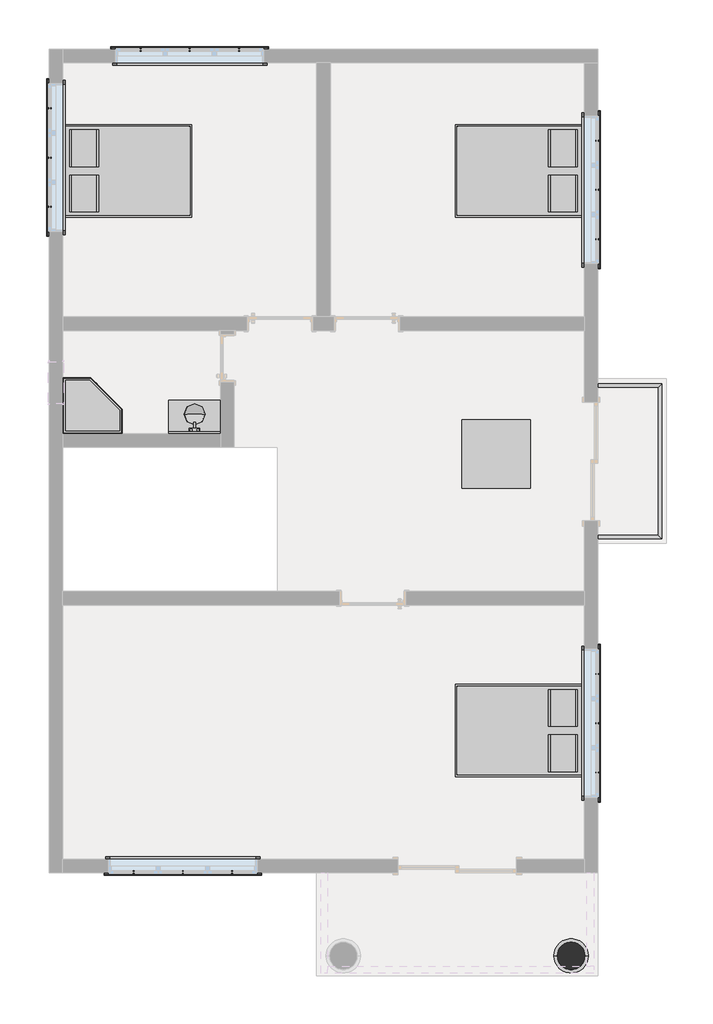
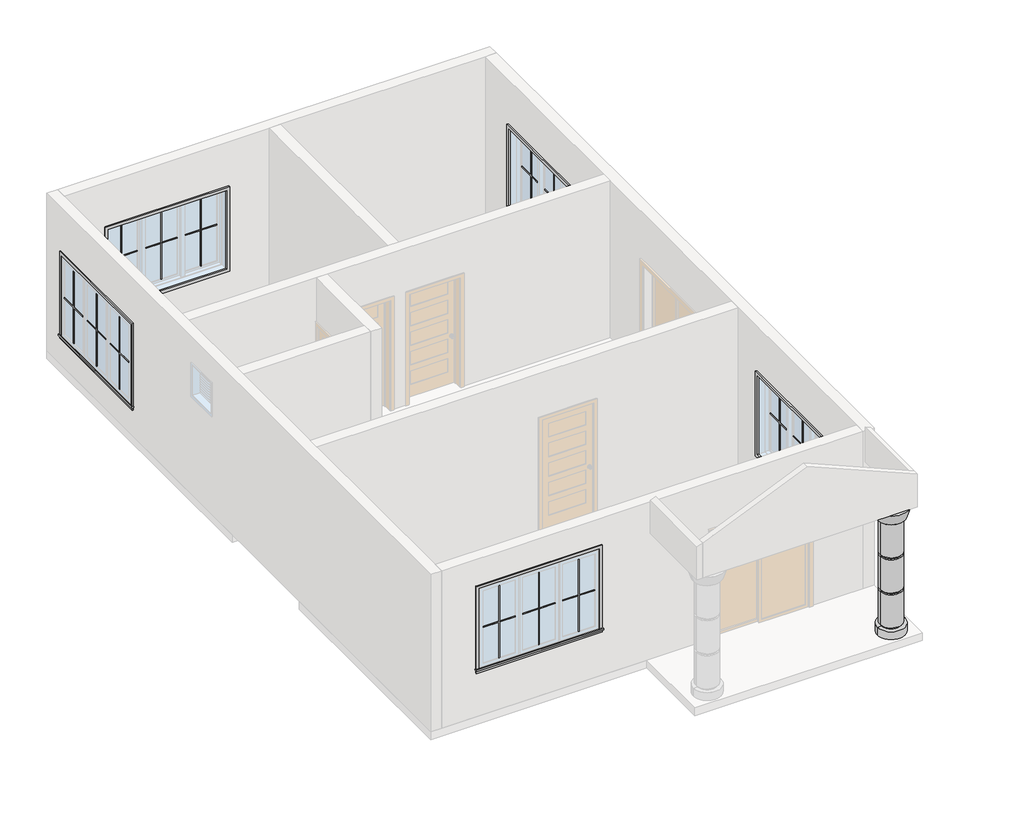
# One storey, part 2 of 2: 25 proxies, 4 furniture elements, 2 flow terminals, 1 column, 1 railing.
"""IFC4 building model written with IfcOpenShell, lengths in millimetres."""

from ifc_helpers import new_model, si_unit, frame, origin, place, context, project, spatial, polyline, circle_curve, outline, extrude, faceted_brep, transform, mapped, element, save
from ifc_brep_helpers import plane_surface, cylinder_surface, revolved_surface, advanced_brep
from components import muntin_pattern_2x2_muntin_pattern_2x2_6849e3ed, muntin_pattern_2x2_muntin_pattern_2x2_a6c43cb1, trim_window_exterior_flat_with_sill_088bf4ff, trim_window_interior_flat_picture_frame_12843d3c, flow_terminal_15267b2a, flow_terminal_2596653b, furniture_1000_x_1000mm_85c88e14, furniture_b58f7881

model = new_model("IFC4")

# Units and contexts
model_context = context("Model", 3, world=origin())
ifc_project = project(units=[si_unit("LENGTHUNIT", "METRE", prefix="MILLI")], contexts=[model_context])

# Site, building, storey
site = spatial("IfcSite", under=ifc_project)
building = spatial("IfcBuilding", under=site)
storey = spatial("IfcBuildingStorey", under=building, Elevation=3400.0)

# Proxies
placement = place(None, origin())
muntin_pattern_2x2_muntin_pattern_2x2_shape = muntin_pattern_2x2_muntin_pattern_2x2_6849e3ed(model_context)
element("IfcBuildingElementProxy", 1, Name="Muntin Pattern_2x2 : Muntin Pattern_2x2", ObjectType="Muntin Pattern_2x2 : Muntin Pattern_2x2", at=placement, inside=storey, context=model_context, shape_type="MappedRepresentation", body=[
    mapped(muntin_pattern_2x2_muntin_pattern_2x2_shape, transform((2649.7091997, -1368.0932863, 4058.55), x_axis=(0.0, -1.0, 0.0), y_axis=(1.0, 0.0, 0.0), z_axis=(0.0, 0.0, 1.0))),
])
element("IfcBuildingElementProxy", 2, Name="Muntin Pattern_2x2 : Muntin Pattern_2x2", ObjectType="Muntin Pattern_2x2 : Muntin Pattern_2x2", at=placement, inside=storey, context=model_context, shape_type="MappedRepresentation", body=[
    mapped(muntin_pattern_2x2_muntin_pattern_2x2_shape, transform((-4008.3158003, 7725.3317137, 4058.55), x_axis=(1.0, 0.0, 0.0), y_axis=(0.0, 1.0, 0.0), z_axis=(0.0, 0.0, 1.0))),
])
element("IfcBuildingElementProxy", 3, Name="Muntin Pattern_2x2 : Muntin Pattern_2x2", ObjectType="Muntin Pattern_2x2 : Muntin Pattern_2x2", at=placement, inside=storey, context=model_context, shape_type="MappedRepresentation", body=[
    mapped(muntin_pattern_2x2_muntin_pattern_2x2_shape, transform((-5331.2408003, 5437.8067137, 4058.55), x_axis=(0.0, 1.0, 0.0), y_axis=(-1.0, 0.0, 0.0), z_axis=(0.0, 0.0, 1.0))),
])
element("IfcBuildingElementProxy", 4, Name="Muntin Pattern_2x2 : Muntin Pattern_2x2", ObjectType="Muntin Pattern_2x2 : Muntin Pattern_2x2", at=placement, inside=storey, context=model_context, shape_type="MappedRepresentation", body=[
    mapped(muntin_pattern_2x2_muntin_pattern_2x2_shape, transform((2649.7091997, 6402.4067137, 4058.55), x_axis=(0.0, -1.0, 0.0), y_axis=(1.0, 0.0, 0.0), z_axis=(0.0, 0.0, 1.0))),
])
element("IfcBuildingElementProxy", 5, Name="Muntin Pattern_2x2 : Muntin Pattern_2x2", ObjectType="Muntin Pattern_2x2 : Muntin Pattern_2x2", at=placement, inside=storey, context=model_context, shape_type="MappedRepresentation", body=[
    mapped(muntin_pattern_2x2_muntin_pattern_2x2_shape, transform((-2673.2158003, -4255.6182863, 4384.25), x_axis=(-1.0, 0.0, 0.0), y_axis=(0.0, -1.0, 0.0), z_axis=(0.0, 0.0, 1.0))),
])
muntin_pattern_2x2_muntin_pattern_2x2_2_shape = muntin_pattern_2x2_muntin_pattern_2x2_a6c43cb1(model_context)
element("IfcBuildingElementProxy", 6, Name="Muntin Pattern_2x2 : Muntin Pattern_2x2", ObjectType="Muntin Pattern_2x2 : Muntin Pattern_2x2", at=placement, inside=storey, context=model_context, shape_type="MappedRepresentation", body=[
    mapped(muntin_pattern_2x2_muntin_pattern_2x2_2_shape, transform((2649.7091997, -2803.1932863, 4058.55), x_axis=(0.0, 1.0, 0.0), y_axis=(-1.0, 0.0, 0.0), z_axis=(0.0, 0.0, 1.0))),
])
element("IfcBuildingElementProxy", 7, Name="Muntin Pattern_2x2 : Muntin Pattern_2x2", ObjectType="Muntin Pattern_2x2 : Muntin Pattern_2x2", at=placement, inside=storey, context=model_context, shape_type="MappedRepresentation", body=[
    mapped(muntin_pattern_2x2_muntin_pattern_2x2_2_shape, transform((2649.7091997, -2085.6432863, 4058.55), x_axis=(0.0, 1.0, 0.0), y_axis=(-1.0, 0.0, 0.0), z_axis=(0.0, 0.0, 1.0))),
])
element("IfcBuildingElementProxy", 8, Name="Muntin Pattern_2x2 : Muntin Pattern_2x2", ObjectType="Muntin Pattern_2x2 : Muntin Pattern_2x2", at=placement, inside=storey, context=model_context, shape_type="MappedRepresentation", body=[
    mapped(muntin_pattern_2x2_muntin_pattern_2x2_2_shape, transform((-2573.2158003, 7725.3317137, 4058.55), x_axis=(-1.0, 0.0, 0.0), y_axis=(0.0, -1.0, 0.0), z_axis=(0.0, 0.0, 1.0))),
])
element("IfcBuildingElementProxy", 9, Name="Muntin Pattern_2x2 : Muntin Pattern_2x2", ObjectType="Muntin Pattern_2x2 : Muntin Pattern_2x2", at=placement, inside=storey, context=model_context, shape_type="MappedRepresentation", body=[
    mapped(muntin_pattern_2x2_muntin_pattern_2x2_2_shape, transform((-3290.7658003, 7725.3317137, 4058.55), x_axis=(-1.0, 0.0, 0.0), y_axis=(0.0, -1.0, 0.0), z_axis=(0.0, 0.0, 1.0))),
])
element("IfcBuildingElementProxy", 10, Name="Muntin Pattern_2x2 : Muntin Pattern_2x2", ObjectType="Muntin Pattern_2x2 : Muntin Pattern_2x2", at=placement, inside=storey, context=model_context, shape_type="MappedRepresentation", body=[
    mapped(muntin_pattern_2x2_muntin_pattern_2x2_2_shape, transform((-5331.2408003, 6872.9067137, 4058.55), x_axis=(0.0, -1.0, 0.0), y_axis=(1.0, 0.0, 0.0), z_axis=(0.0, 0.0, 1.0))),
])
element("IfcBuildingElementProxy", 11, Name="Muntin Pattern_2x2 : Muntin Pattern_2x2", ObjectType="Muntin Pattern_2x2 : Muntin Pattern_2x2", at=placement, inside=storey, context=model_context, shape_type="MappedRepresentation", body=[
    mapped(muntin_pattern_2x2_muntin_pattern_2x2_2_shape, transform((-5331.2408003, 6155.3567137, 4058.55), x_axis=(0.0, -1.0, 0.0), y_axis=(1.0, 0.0, 0.0), z_axis=(0.0, 0.0, 1.0))),
])
element("IfcBuildingElementProxy", 12, Name="Muntin Pattern_2x2 : Muntin Pattern_2x2", ObjectType="Muntin Pattern_2x2 : Muntin Pattern_2x2", at=placement, inside=storey, context=model_context, shape_type="MappedRepresentation", body=[
    mapped(muntin_pattern_2x2_muntin_pattern_2x2_2_shape, transform((2649.7091997, 4967.3067137, 4058.55), x_axis=(0.0, 1.0, 0.0), y_axis=(-1.0, 0.0, 0.0), z_axis=(0.0, 0.0, 1.0))),
])
element("IfcBuildingElementProxy", 13, Name="Muntin Pattern_2x2 : Muntin Pattern_2x2", ObjectType="Muntin Pattern_2x2 : Muntin Pattern_2x2", at=placement, inside=storey, context=model_context, shape_type="MappedRepresentation", body=[
    mapped(muntin_pattern_2x2_muntin_pattern_2x2_2_shape, transform((2649.7091997, 5684.8567137, 4058.55), x_axis=(0.0, 1.0, 0.0), y_axis=(-1.0, 0.0, 0.0), z_axis=(0.0, 0.0, 1.0))),
])
element("IfcBuildingElementProxy", 14, Name="Muntin Pattern_2x2 : Muntin Pattern_2x2", ObjectType="Muntin Pattern_2x2 : Muntin Pattern_2x2", at=placement, inside=storey, context=model_context, shape_type="MappedRepresentation", body=[
    mapped(muntin_pattern_2x2_muntin_pattern_2x2_2_shape, transform((-4108.3158003, -4255.6182863, 4384.25), x_axis=(1.0, 0.0, 0.0), y_axis=(0.0, 1.0, 0.0), z_axis=(0.0, 0.0, 1.0))),
])
element("IfcBuildingElementProxy", 15, Name="Muntin Pattern_2x2 : Muntin Pattern_2x2", ObjectType="Muntin Pattern_2x2 : Muntin Pattern_2x2", at=placement, inside=storey, context=model_context, shape_type="MappedRepresentation", body=[
    mapped(muntin_pattern_2x2_muntin_pattern_2x2_2_shape, transform((-3390.7658003, -4255.6182863, 4384.25), x_axis=(1.0, 0.0, 0.0), y_axis=(0.0, 1.0, 0.0), z_axis=(0.0, 0.0, 1.0))),
])
trim_window_exterior_flat_with_sill_shape = trim_window_exterior_flat_with_sill_088bf4ff(model_context)
element("IfcBuildingElementProxy", 16, Name="Trim-Window-Exterior-Flat : with Sill", ObjectType="Trim-Window-Exterior-Flat : with Sill", at=placement, inside=storey, context=model_context, shape_type="MappedRepresentation", body=[
    mapped(trim_window_exterior_flat_with_sill_shape, transform((2659.2341997, -2085.6432863, 5512.7), x_axis=(0.0, 1.0, 0.0), y_axis=(0.0, 0.0, 1.0), z_axis=(1.0, 0.0, 0.0))),
])
element("IfcBuildingElementProxy", 17, Name="Trim-Window-Exterior-Flat : with Sill", ObjectType="Trim-Window-Exterior-Flat : with Sill", at=placement, inside=storey, context=model_context, shape_type="MappedRepresentation", body=[
    mapped(trim_window_exterior_flat_with_sill_shape, transform((-3290.7658003, 7734.8567137, 5512.7), x_axis=(-1.0, 0.0, 0.0), y_axis=(0.0, 0.0, 1.0), z_axis=(0.0, 1.0, 0.0))),
])
element("IfcBuildingElementProxy", 18, Name="Trim-Window-Exterior-Flat : with Sill", ObjectType="Trim-Window-Exterior-Flat : with Sill", at=placement, inside=storey, context=model_context, shape_type="MappedRepresentation", body=[
    mapped(trim_window_exterior_flat_with_sill_shape, transform((-5340.7658003, 6155.3567137, 5512.7), x_axis=(0.0, -1.0, 0.0), y_axis=(0.0, 0.0, 1.0), z_axis=(-1.0, 0.0, 0.0))),
])
element("IfcBuildingElementProxy", 19, Name="Trim-Window-Exterior-Flat : with Sill", ObjectType="Trim-Window-Exterior-Flat : with Sill", at=placement, inside=storey, context=model_context, shape_type="MappedRepresentation", body=[
    mapped(trim_window_exterior_flat_with_sill_shape, transform((2659.2341997, 5684.8567137, 5512.7), x_axis=(0.0, 1.0, 0.0), y_axis=(0.0, 0.0, 1.0), z_axis=(1.0, 0.0, 0.0))),
])
element("IfcBuildingElementProxy", 20, Name="Trim-Window-Exterior-Flat : with Sill", ObjectType="Trim-Window-Exterior-Flat : with Sill", at=placement, inside=storey, context=model_context, shape_type="MappedRepresentation", body=[
    mapped(trim_window_exterior_flat_with_sill_shape, transform((-3390.7658003, -4265.1432863, 5838.4), x_axis=(1.0, 0.0, 0.0), y_axis=(0.0, 0.0, 1.0), z_axis=(0.0, -1.0, 0.0))),
])
trim_window_interior_flat_picture_frame_shape = trim_window_interior_flat_picture_frame_12843d3c(model_context)
element("IfcBuildingElementProxy", 21, Name="Trim-Window-Interior-Flat : Picture Frame", ObjectType="Trim-Window-Interior-Flat : Picture Frame", at=placement, inside=storey, context=model_context, shape_type="MappedRepresentation", body=[
    mapped(trim_window_interior_flat_picture_frame_shape, transform((2459.2341997, -2085.6432863, 5512.7), x_axis=(0.0, -1.0, 0.0), y_axis=(0.0, 0.0, 1.0), z_axis=(-1.0, 0.0, 0.0))),
])
element("IfcBuildingElementProxy", 22, Name="Trim-Window-Interior-Flat : Picture Frame", ObjectType="Trim-Window-Interior-Flat : Picture Frame", at=placement, inside=storey, context=model_context, shape_type="MappedRepresentation", body=[
    mapped(trim_window_interior_flat_picture_frame_shape, transform((-3290.7658003, 7534.8567137, 5512.7), x_axis=(1.0, 0.0, 0.0), y_axis=(0.0, 0.0, 1.0), z_axis=(0.0, -1.0, 0.0))),
])
element("IfcBuildingElementProxy", 23, Name="Trim-Window-Interior-Flat : Picture Frame", ObjectType="Trim-Window-Interior-Flat : Picture Frame", at=placement, inside=storey, context=model_context, shape_type="MappedRepresentation", body=[
    mapped(trim_window_interior_flat_picture_frame_shape, transform((-5140.7658003, 6155.3567137, 5512.7), x_axis=(0.0, 1.0, 0.0), y_axis=(0.0, 0.0, 1.0), z_axis=(1.0, 0.0, 0.0))),
])
element("IfcBuildingElementProxy", 24, Name="Trim-Window-Interior-Flat : Picture Frame", ObjectType="Trim-Window-Interior-Flat : Picture Frame", at=placement, inside=storey, context=model_context, shape_type="MappedRepresentation", body=[
    mapped(trim_window_interior_flat_picture_frame_shape, transform((2459.2341997, 5684.8567137, 5512.7), x_axis=(0.0, -1.0, 0.0), y_axis=(0.0, 0.0, 1.0), z_axis=(-1.0, 0.0, 0.0))),
])
element("IfcBuildingElementProxy", 25, Name="Trim-Window-Interior-Flat : Picture Frame", ObjectType="Trim-Window-Interior-Flat : Picture Frame", at=placement, inside=storey, context=model_context, shape_type="MappedRepresentation", body=[
    mapped(trim_window_interior_flat_picture_frame_shape, transform((-3390.7658003, -4065.1432863, 5838.4), x_axis=(-1.0, 0.0, 0.0), y_axis=(0.0, 0.0, 1.0), z_axis=(0.0, 1.0, 0.0))),
])

# Column
element("IfcColumn", 26, ObjectType="Metal Clad Column : 400MM COLUMN", at=placement, inside=storey, context=model_context, shape_type="AdvancedBrep", body=[
    advanced_brep(
    [(2269.2341997, -5475.1432863, 3400.0), (2018.4341997, -5475.1432863, 3400.0), (2520.0341997, -5475.1432863, 3400.0), (2018.4341997, -5475.1432863, 3552.4), (2520.0341997, -5475.1432863, 3552.4), (2094.6341997, -5475.1432863, 4259.2666667), (2069.2341997, -5475.1432863, 4259.2666667), (2469.2341997, -5475.1432863, 4259.2666667), (2443.8341997, -5475.1432863, 4259.2666667), (2069.2341997, -5475.1432863, 4889.9333333), (2469.2341997, -5475.1432863, 4889.9333333), (2094.6341997, -5475.1432863, 4221.1666667), (2443.8341997, -5475.1432863, 4221.1666667), (2069.2341997, -5475.1432863, 4221.1666667), (2469.2341997, -5475.1432863, 4221.1666667), (2069.2341997, -5475.1432863, 3590.5), (2469.2341997, -5475.1432863, 3590.5), (2094.6341997, -5475.1432863, 3590.5), (2443.8341997, -5475.1432863, 3590.5), (2094.6341997, -5475.1432863, 3552.4), (2443.8341997, -5475.1432863, 3552.4), (2018.4341997, -5475.1432863, 5596.8), (1954.9341997, -5475.1432863, 5800.0), (2583.5341997, -5475.1432863, 5800.0), (2520.0341997, -5475.1432863, 5596.8), (2269.2341997, -5475.1432863, 5800.0), (2094.6341997, -5475.1432863, 5596.8), (2443.8341997, -5475.1432863, 5596.8), (2094.6341997, -5475.1432863, 5558.7), (2443.8341997, -5475.1432863, 5558.7), (2069.2341997, -5475.1432863, 5558.7), (2469.2341997, -5475.1432863, 5558.7), (2069.2341997, -5475.1432863, 4928.0333333), (2469.2341997, -5475.1432863, 4928.0333333), (2094.6341997, -5475.1432863, 4928.0333333), (2443.8341997, -5475.1432863, 4928.0333333), (2094.6341997, -5475.1432863, 4889.9333333), (2443.8341997, -5475.1432863, 4889.9333333)],
    [
        (0, 1),
        (1, 2, circle_curve(frame((2269.2341997, -5475.1432863, 3400.0), z_axis=(0.0, 0.0, -1.0), x_axis=(1.0, 0.0, 0.0)), 250.8)),
        (2, 0),
        (2, 1, circle_curve(frame((2269.2341997, -5475.1432863, 3400.0), z_axis=(0.0, 0.0, -1.0), x_axis=(1.0, 0.0, 0.0)), 250.8)),
        (1, 3),
        (3, 4, circle_curve(frame((2269.2341997, -5475.1432863, 3552.4), z_axis=(0.0, 0.0, -1.0), x_axis=(1.0, 0.0, 0.0)), 250.8)),
        (4, 2),
        (4, 3, circle_curve(frame((2269.2341997, -5475.1432863, 3552.4), z_axis=(0.0, 0.0, -1.0), x_axis=(1.0, 0.0, 0.0)), 250.8)),
        (5, 6),
        (6, 7, circle_curve(frame((2269.2341997, -5475.1432863, 4259.2666667), z_axis=(0.0, 0.0, -1.0), x_axis=(1.0, 0.0, 0.0)), 200.0)),
        (7, 8),
        (8, 5, circle_curve(frame((2269.2341997, -5475.1432863, 4259.2666667), z_axis=(0.0, 0.0, 1.0), x_axis=(1.0, 0.0, 0.0)), 174.6)),
        (6, 9),
        (9, 10, circle_curve(frame((2269.2341997, -5475.1432863, 4889.9333333), z_axis=(0.0, 0.0, -1.0), x_axis=(1.0, 0.0, 0.0)), 200.0)),
        (10, 7),
        (10, 9, circle_curve(frame((2269.2341997, -5475.1432863, 4889.9333333), z_axis=(0.0, 0.0, -1.0), x_axis=(1.0, 0.0, 0.0)), 200.0)),
        (6, 7, circle_curve(frame((2269.2341997, -5475.1432863, 4259.2666667), z_axis=(0.0, 0.0, 1.0), x_axis=(1.0, 0.0, 0.0)), 200.0)),
        (5, 8, circle_curve(frame((2269.2341997, -5475.1432863, 4259.2666667), z_axis=(0.0, 0.0, 1.0), x_axis=(1.0, 0.0, 0.0)), 174.6)),
        (11, 5),
        (8, 12),
        (12, 11, circle_curve(frame((2269.2341997, -5475.1432863, 4221.1666667), z_axis=(0.0, 0.0, 1.0), x_axis=(1.0, 0.0, 0.0)), 174.6)),
        (11, 12, circle_curve(frame((2269.2341997, -5475.1432863, 4221.1666667), z_axis=(0.0, 0.0, 1.0), x_axis=(1.0, 0.0, 0.0)), 174.6)),
        (13, 11),
        (12, 14),
        (14, 13, circle_curve(frame((2269.2341997, -5475.1432863, 4221.1666667), z_axis=(0.0, 0.0, 1.0), x_axis=(1.0, 0.0, 0.0)), 200.0)),
        (13, 14, circle_curve(frame((2269.2341997, -5475.1432863, 4221.1666667), z_axis=(0.0, 0.0, 1.0), x_axis=(1.0, 0.0, 0.0)), 200.0)),
        (15, 13),
        (14, 16),
        (16, 15, circle_curve(frame((2269.2341997, -5475.1432863, 3590.5), z_axis=(0.0, 0.0, 1.0), x_axis=(1.0, 0.0, 0.0)), 200.0)),
        (15, 16, circle_curve(frame((2269.2341997, -5475.1432863, 3590.5), z_axis=(0.0, 0.0, 1.0), x_axis=(1.0, 0.0, 0.0)), 200.0)),
        (17, 15),
        (16, 18),
        (18, 17, circle_curve(frame((2269.2341997, -5475.1432863, 3590.5), z_axis=(0.0, 0.0, 1.0), x_axis=(1.0, 0.0, 0.0)), 174.6)),
        (17, 18, circle_curve(frame((2269.2341997, -5475.1432863, 3590.5), z_axis=(0.0, 0.0, 1.0), x_axis=(1.0, 0.0, 0.0)), 174.6)),
        (19, 17),
        (18, 20),
        (20, 19, circle_curve(frame((2269.2341997, -5475.1432863, 3552.4), z_axis=(0.0, 0.0, 1.0), x_axis=(1.0, 0.0, 0.0)), 174.6)),
        (19, 20, circle_curve(frame((2269.2341997, -5475.1432863, 3552.4), z_axis=(0.0, 0.0, 1.0), x_axis=(1.0, 0.0, 0.0)), 174.6)),
        (3, 19),
        (20, 4),
        (21, 22),
        (22, 23, circle_curve(frame((2269.2341997, -5475.1432863, 5800.0), z_axis=(0.0, 0.0, -1.0), x_axis=(1.0, 0.0, 0.0)), 314.3)),
        (23, 24),
        (24, 21, circle_curve(frame((2269.2341997, -5475.1432863, 5596.8), z_axis=(0.0, 0.0, 1.0), x_axis=(1.0, 0.0, 0.0)), 250.8)),
        (22, 25),
        (25, 23),
        (22, 23, circle_curve(frame((2269.2341997, -5475.1432863, 5800.0), z_axis=(0.0, 0.0, 1.0), x_axis=(1.0, 0.0, 0.0)), 314.3)),
        (21, 24, circle_curve(frame((2269.2341997, -5475.1432863, 5596.8), z_axis=(0.0, 0.0, 1.0), x_axis=(1.0, 0.0, 0.0)), 250.8)),
        (26, 21),
        (24, 27),
        (27, 26, circle_curve(frame((2269.2341997, -5475.1432863, 5596.8), z_axis=(0.0, 0.0, 1.0), x_axis=(1.0, 0.0, 0.0)), 174.6)),
        (26, 27, circle_curve(frame((2269.2341997, -5475.1432863, 5596.8), z_axis=(0.0, 0.0, 1.0), x_axis=(1.0, 0.0, 0.0)), 174.6)),
        (28, 26),
        (27, 29),
        (29, 28, circle_curve(frame((2269.2341997, -5475.1432863, 5558.7), z_axis=(0.0, 0.0, 1.0), x_axis=(1.0, 0.0, 0.0)), 174.6)),
        (28, 29, circle_curve(frame((2269.2341997, -5475.1432863, 5558.7), z_axis=(0.0, 0.0, 1.0), x_axis=(1.0, 0.0, 0.0)), 174.6)),
        (30, 28),
        (29, 31),
        (31, 30, circle_curve(frame((2269.2341997, -5475.1432863, 5558.7), z_axis=(0.0, 0.0, 1.0), x_axis=(1.0, 0.0, 0.0)), 200.0)),
        (30, 31, circle_curve(frame((2269.2341997, -5475.1432863, 5558.7), z_axis=(0.0, 0.0, 1.0), x_axis=(1.0, 0.0, 0.0)), 200.0)),
        (32, 30),
        (31, 33),
        (33, 32, circle_curve(frame((2269.2341997, -5475.1432863, 4928.0333333), z_axis=(0.0, 0.0, 1.0), x_axis=(1.0, 0.0, 0.0)), 200.0)),
        (32, 33, circle_curve(frame((2269.2341997, -5475.1432863, 4928.0333333), z_axis=(0.0, 0.0, 1.0), x_axis=(1.0, 0.0, 0.0)), 200.0)),
        (34, 32),
        (33, 35),
        (35, 34, circle_curve(frame((2269.2341997, -5475.1432863, 4928.0333333), z_axis=(0.0, 0.0, 1.0), x_axis=(1.0, 0.0, 0.0)), 174.6)),
        (34, 35, circle_curve(frame((2269.2341997, -5475.1432863, 4928.0333333), z_axis=(0.0, 0.0, 1.0), x_axis=(1.0, 0.0, 0.0)), 174.6)),
        (36, 34),
        (35, 37),
        (37, 36, circle_curve(frame((2269.2341997, -5475.1432863, 4889.9333333), z_axis=(0.0, 0.0, 1.0), x_axis=(1.0, 0.0, 0.0)), 174.6)),
        (36, 37, circle_curve(frame((2269.2341997, -5475.1432863, 4889.9333333), z_axis=(0.0, 0.0, 1.0), x_axis=(1.0, 0.0, 0.0)), 174.6)),
        (9, 36),
        (37, 10),
    ],
    [
        plane_surface(frame((2269.2341997, -5475.1432863, 3400.0), z_axis=(0.0, 0.0, -1.0), x_axis=(1.0, 0.0, 0.0))),
        cylinder_surface(frame((2269.2341997, -5475.1432863, 5800.0), z_axis=(0.0, 0.0, -1.0), x_axis=(1.0, 0.0, 0.0)), 250.8),
        plane_surface(frame((2269.2341997, -5475.1432863, 4259.2666667), z_axis=(0.0, 0.0, -1.0), x_axis=(1.0, 0.0, 0.0))),
        cylinder_surface(frame((2269.2341997, -5475.1432863, 5800.0), z_axis=(0.0, 0.0, -1.0), x_axis=(1.0, 0.0, 0.0)), 200.0),
        cylinder_surface(frame((2269.2341997, -5475.1432863, 5800.0), z_axis=(0.0, 0.0, -1.0), x_axis=(1.0, 0.0, 0.0)), 174.6),
        plane_surface(frame((2269.2341997, -5475.1432863, 4221.1666667), z_axis=(0.0, 0.0, 1.0), x_axis=(1.0, 0.0, 0.0))),
        plane_surface(frame((2269.2341997, -5475.1432863, 3590.5), z_axis=(0.0, 0.0, -1.0), x_axis=(1.0, 0.0, 0.0))),
        plane_surface(frame((2269.2341997, -5475.1432863, 3552.4), z_axis=(0.0, 0.0, 1.0), x_axis=(1.0, 0.0, 0.0))),
        revolved_surface(polyline([(2583.5341997, -5475.1432863, 5800.0), (2520.0341997, -5475.1432863, 5596.8)]), (2269.2341997, -5475.1432863, 5800.0), (0.0, 0.0, -1.0)),
        plane_surface(frame((2269.2341997, -5475.1432863, 5800.0), z_axis=(0.0, 0.0, 1.0), x_axis=(1.0, 0.0, 0.0))),
        plane_surface(frame((2269.2341997, -5475.1432863, 5596.8), z_axis=(0.0, 0.0, -1.0), x_axis=(1.0, 0.0, 0.0))),
        plane_surface(frame((2269.2341997, -5475.1432863, 5558.7), z_axis=(0.0, 0.0, 1.0), x_axis=(1.0, 0.0, 0.0))),
        plane_surface(frame((2269.2341997, -5475.1432863, 4928.0333333), z_axis=(0.0, 0.0, -1.0), x_axis=(1.0, 0.0, 0.0))),
        plane_surface(frame((2269.2341997, -5475.1432863, 4889.9333333), z_axis=(0.0, 0.0, 1.0), x_axis=(1.0, 0.0, 0.0))),
    ],
    [
        (0, [[1, 2, 3]]),
        (0, [[-3, 4, -1]]),
        (1, [[5, 6, 7, -2]]),
        (1, [[-7, 8, -5, -4]]),
        (2, [[9, 10, 11, 12]]),
        (3, [[13, 14, 15, -10]]),
        (3, [[-15, 16, -13, 17]]),
        (2, [[-11, -17, -9, 18]]),
        (4, [[19, -12, 20, 21]]),
        (4, [[-20, -18, -19, 22]]),
        (5, [[23, -21, 24, 25]]),
        (5, [[-24, -22, -23, 26]]),
        (3, [[27, -25, 28, 29]]),
        (3, [[-28, -26, -27, 30]]),
        (6, [[31, -29, 32, 33]]),
        (6, [[-32, -30, -31, 34]]),
        (4, [[35, -33, 36, 37]]),
        (4, [[-36, -34, -35, 38]]),
        (7, [[39, -37, 40, -6]]),
        (7, [[-40, -38, -39, -8]]),
        (8, [[41, 42, 43, 44]]),
        (9, [[45, 46, -42]]),
        (9, [[-46, -45, 47]]),
        (8, [[-43, -47, -41, 48]]),
        (10, [[49, -44, 50, 51]]),
        (10, [[-50, -48, -49, 52]]),
        (4, [[53, -51, 54, 55]]),
        (4, [[-54, -52, -53, 56]]),
        (11, [[57, -55, 58, 59]]),
        (11, [[-58, -56, -57, 60]]),
        (3, [[61, -59, 62, 63]]),
        (3, [[-62, -60, -61, 64]]),
        (12, [[65, -63, 66, 67]]),
        (12, [[-66, -64, -65, 68]]),
        (4, [[69, -67, 70, 71]]),
        (4, [[-70, -68, -69, 72]]),
        (13, [[73, -71, 74, -14]]),
        (13, [[-74, -72, -73, -16]]),
    ],
),
])

# Flow terminals
flow_terminal_shape = flow_terminal_15267b2a(model_context)
element("IfcFlowTerminal", 27, ObjectType="Lavatory - Vanity : 30\"x18\" - Public", at=placement, inside=storey, context=model_context, shape_type="MappedRepresentation", body=[
    mapped(flow_terminal_shape, transform((-3220.7658003, 2134.8567137, 3400.0), x_axis=(0.0, 1.0, 0.0), y_axis=(-1.0, 0.0, 0.0), z_axis=(0.0, 0.0, 1.0))),
])
flow_terminal_2_shape = flow_terminal_2596653b(model_context)
element("IfcFlowTerminal", 28, ObjectType="Shower Stall - Corner : 34\"x32\" - Private", at=placement, inside=storey, context=model_context, shape_type="MappedRepresentation", body=[
    mapped(flow_terminal_2_shape, transform((-5140.7658003, 2134.8567137, 3400.0), x_axis=(1.0, 0.0, 0.0), y_axis=(0.0, 1.0, 0.0), z_axis=(0.0, 0.0, 1.0))),
])

# Furniture
furniture_1000_x_1000mm_shape = furniture_1000_x_1000mm_85c88e14(model_context)
element("IfcFurniture", 29, ObjectType="1000 x 1000mm", at=placement, inside=storey, context=model_context, shape_type="MappedRepresentation", body=[
    mapped(furniture_1000_x_1000mm_shape, transform((1232.8145276, 1894.8044789, 3400.0), x_axis=(1.0, 0.0, 0.0), y_axis=(0.0, 1.0, 0.0), z_axis=(0.0, 0.0, 1.0))),
])
furniture_shape = furniture_b58f7881(model_context)
element("IfcFurniture", 30, ObjectType="Bed-Box : Double 53\" x 74\"", at=placement, inside=storey, context=model_context, shape_type="MappedRepresentation", body=[
    mapped(furniture_shape, transform((-4435.3953085, 5622.6042547, 3400.0), x_axis=(0.0, 1.0, 0.0), y_axis=(-1.0, 0.0, 0.0), z_axis=(0.0, 0.0, 1.0))),
])
element("IfcFurniture", 31, ObjectType="Bed-Box : Double 53\" x 74\"", at=placement, inside=storey, context=model_context, shape_type="MappedRepresentation", body=[
    mapped(furniture_shape, transform((1753.8637079, 6300.9091728, 3400.0), x_axis=(0.0, -1.0, 0.0), y_axis=(1.0, 0.0, 0.0), z_axis=(0.0, 0.0, 1.0))),
])
element("IfcFurniture", 32, ObjectType="Bed-Box : Double 53\" x 74\"", at=placement, inside=storey, context=model_context, shape_type="MappedRepresentation", body=[
    mapped(furniture_shape, transform((1753.8637079, -1852.8908272, 3400.0), x_axis=(0.0, -1.0, 0.0), y_axis=(1.0, 0.0, 0.0), z_axis=(0.0, 0.0, 1.0))),
])

# Railing
element("IfcRailing", 33, ObjectType="Handrail - Rectangular", at=placement, inside=storey, context=model_context, shape_type="SolidModel", body=[
    faceted_brep([(2659.2341997, 2860.2567137, 4314.4), (2659.2341997, 2860.2567137, 4263.6), (2659.2341997, 2809.4567137, 4263.6), (2659.2341997, 2809.4567137, 4314.4), (3589.6341997, 2860.2567137, 4314.4), (3589.6341997, 2860.2567137, 4263.6), (3538.8341997, 2809.4567137, 4263.6), (3538.8341997, 2809.4567137, 4314.4), (3589.6341997, 604.4567137, 4314.4), (3589.6341997, 604.4567137, 4263.6), (3538.8341997, 655.2567137, 4263.6), (3538.8341997, 655.2567137, 4314.4), (2659.2341997, 604.4567137, 4314.4), (2659.2341997, 655.2567137, 4314.4), (2659.2341997, 655.2567137, 4263.6), (2659.2341997, 604.4567137, 4263.6)], [[[0, 1, 2, 3]], [[1, 0, 4, 5]], [[2, 1, 5, 6]], [[3, 2, 6, 7]], [[0, 3, 7, 4]], [[5, 4, 8, 9]], [[6, 5, 9, 10]], [[7, 6, 10, 11]], [[4, 7, 11, 8]], [[12, 13, 14, 15]], [[9, 8, 12, 15]], [[10, 9, 15, 14]], [[11, 10, 14, 13]], [[8, 11, 13, 12]]]),
    extrude(outline(polyline([(2760.9591997, 639.3817137), (2760.9591997, 620.3317137), (2741.9091997, 620.3317137), (2741.9091997, 639.3817137), (2760.9591997, 639.3817137)])), frame((0.0, 0.0, 3400.0), z_axis=(0.0, 0.0, 1.0), x_axis=(1.0, 0.0, 0.0)), (0.0, 0.0, 1.0), 863.6),
    extrude(outline(polyline([(2862.5591997, 639.3817137), (2862.5591997, 620.3317137), (2843.5091997, 620.3317137), (2843.5091997, 639.3817137), (2862.5591997, 639.3817137)])), frame((0.0, 0.0, 3400.0), z_axis=(0.0, 0.0, 1.0), x_axis=(1.0, 0.0, 0.0)), (0.0, 0.0, 1.0), 863.6),
    extrude(outline(polyline([(2964.1591997, 639.3817137), (2964.1591997, 620.3317137), (2945.1091997, 620.3317137), (2945.1091997, 639.3817137), (2964.1591997, 639.3817137)])), frame((0.0, 0.0, 3400.0), z_axis=(0.0, 0.0, 1.0), x_axis=(1.0, 0.0, 0.0)), (0.0, 0.0, 1.0), 863.6),
    extrude(outline(polyline([(3065.7591997, 639.3817137), (3065.7591997, 620.3317137), (3046.7091997, 620.3317137), (3046.7091997, 639.3817137), (3065.7591997, 639.3817137)])), frame((0.0, 0.0, 3400.0), z_axis=(0.0, 0.0, 1.0), x_axis=(1.0, 0.0, 0.0)), (0.0, 0.0, 1.0), 863.6),
    extrude(outline(polyline([(3167.3591997, 639.3817137), (3167.3591997, 620.3317137), (3148.3091997, 620.3317137), (3148.3091997, 639.3817137), (3167.3591997, 639.3817137)])), frame((0.0, 0.0, 3400.0), z_axis=(0.0, 0.0, 1.0), x_axis=(1.0, 0.0, 0.0)), (0.0, 0.0, 1.0), 863.6),
    extrude(outline(polyline([(3268.9591997, 639.3817137), (3268.9591997, 620.3317137), (3249.9091997, 620.3317137), (3249.9091997, 639.3817137), (3268.9591997, 639.3817137)])), frame((0.0, 0.0, 3400.0), z_axis=(0.0, 0.0, 1.0), x_axis=(1.0, 0.0, 0.0)), (0.0, 0.0, 1.0), 863.6),
    extrude(outline(polyline([(3370.5591997, 639.3817137), (3370.5591997, 620.3317137), (3351.5091997, 620.3317137), (3351.5091997, 639.3817137), (3370.5591997, 639.3817137)])), frame((0.0, 0.0, 3400.0), z_axis=(0.0, 0.0, 1.0), x_axis=(1.0, 0.0, 0.0)), (0.0, 0.0, 1.0), 863.6),
    extrude(outline(polyline([(3472.1591997, 639.3817137), (3472.1591997, 620.3317137), (3453.1091997, 620.3317137), (3453.1091997, 639.3817137), (3472.1591997, 639.3817137)])), frame((0.0, 0.0, 3400.0), z_axis=(0.0, 0.0, 1.0), x_axis=(1.0, 0.0, 0.0)), (0.0, 0.0, 1.0), 863.6),
    extrude(outline(polyline([(3554.7091997, 710.7817137), (3573.7591997, 710.7817137), (3573.7591997, 691.7317137), (3554.7091997, 691.7317137), (3554.7091997, 710.7817137)])), frame((0.0, 0.0, 3400.0), z_axis=(0.0, 0.0, 1.0), x_axis=(1.0, 0.0, 0.0)), (0.0, 0.0, 1.0), 863.6),
    extrude(outline(polyline([(3554.7091997, 812.3817137), (3573.7591997, 812.3817137), (3573.7591997, 793.3317137), (3554.7091997, 793.3317137), (3554.7091997, 812.3817137)])), frame((0.0, 0.0, 3400.0), z_axis=(0.0, 0.0, 1.0), x_axis=(1.0, 0.0, 0.0)), (0.0, 0.0, 1.0), 863.6),
    extrude(outline(polyline([(3554.7091997, 913.9817137), (3573.7591997, 913.9817137), (3573.7591997, 894.9317137), (3554.7091997, 894.9317137), (3554.7091997, 913.9817137)])), frame((0.0, 0.0, 3400.0), z_axis=(0.0, 0.0, 1.0), x_axis=(1.0, 0.0, 0.0)), (0.0, 0.0, 1.0), 863.6),
    extrude(outline(polyline([(3554.7091997, 1015.5817137), (3573.7591997, 1015.5817137), (3573.7591997, 996.5317137), (3554.7091997, 996.5317137), (3554.7091997, 1015.5817137)])), frame((0.0, 0.0, 3400.0), z_axis=(0.0, 0.0, 1.0), x_axis=(1.0, 0.0, 0.0)), (0.0, 0.0, 1.0), 863.6),
    extrude(outline(polyline([(3554.7091997, 1117.1817137), (3573.7591997, 1117.1817137), (3573.7591997, 1098.1317137), (3554.7091997, 1098.1317137), (3554.7091997, 1117.1817137)])), frame((0.0, 0.0, 3400.0), z_axis=(0.0, 0.0, 1.0), x_axis=(1.0, 0.0, 0.0)), (0.0, 0.0, 1.0), 863.6),
    extrude(outline(polyline([(3554.7091997, 1218.7817137), (3573.7591997, 1218.7817137), (3573.7591997, 1199.7317137), (3554.7091997, 1199.7317137), (3554.7091997, 1218.7817137)])), frame((0.0, 0.0, 3400.0), z_axis=(0.0, 0.0, 1.0), x_axis=(1.0, 0.0, 0.0)), (0.0, 0.0, 1.0), 863.6),
    extrude(outline(polyline([(3554.7091997, 1320.3817137), (3573.7591997, 1320.3817137), (3573.7591997, 1301.3317137), (3554.7091997, 1301.3317137), (3554.7091997, 1320.3817137)])), frame((0.0, 0.0, 3400.0), z_axis=(0.0, 0.0, 1.0), x_axis=(1.0, 0.0, 0.0)), (0.0, 0.0, 1.0), 863.6),
    extrude(outline(polyline([(3554.7091997, 1421.9817137), (3573.7591997, 1421.9817137), (3573.7591997, 1402.9317137), (3554.7091997, 1402.9317137), (3554.7091997, 1421.9817137)])), frame((0.0, 0.0, 3400.0), z_axis=(0.0, 0.0, 1.0), x_axis=(1.0, 0.0, 0.0)), (0.0, 0.0, 1.0), 863.6),
    extrude(outline(polyline([(3554.7091997, 1523.5817137), (3573.7591997, 1523.5817137), (3573.7591997, 1504.5317137), (3554.7091997, 1504.5317137), (3554.7091997, 1523.5817137)])), frame((0.0, 0.0, 3400.0), z_axis=(0.0, 0.0, 1.0), x_axis=(1.0, 0.0, 0.0)), (0.0, 0.0, 1.0), 863.6),
    extrude(outline(polyline([(3554.7091997, 1625.1817137), (3573.7591997, 1625.1817137), (3573.7591997, 1606.1317137), (3554.7091997, 1606.1317137), (3554.7091997, 1625.1817137)])), frame((0.0, 0.0, 3400.0), z_axis=(0.0, 0.0, 1.0), x_axis=(1.0, 0.0, 0.0)), (0.0, 0.0, 1.0), 863.6),
    extrude(outline(polyline([(3554.7091997, 1726.7817137), (3573.7591997, 1726.7817137), (3573.7591997, 1707.7317137), (3554.7091997, 1707.7317137), (3554.7091997, 1726.7817137)])), frame((0.0, 0.0, 3400.0), z_axis=(0.0, 0.0, 1.0), x_axis=(1.0, 0.0, 0.0)), (0.0, 0.0, 1.0), 863.6),
    extrude(outline(polyline([(3554.7091997, 1828.3817137), (3573.7591997, 1828.3817137), (3573.7591997, 1809.3317137), (3554.7091997, 1809.3317137), (3554.7091997, 1828.3817137)])), frame((0.0, 0.0, 3400.0), z_axis=(0.0, 0.0, 1.0), x_axis=(1.0, 0.0, 0.0)), (0.0, 0.0, 1.0), 863.6),
    extrude(outline(polyline([(3554.7091997, 1929.9817137), (3573.7591997, 1929.9817137), (3573.7591997, 1910.9317137), (3554.7091997, 1910.9317137), (3554.7091997, 1929.9817137)])), frame((0.0, 0.0, 3400.0), z_axis=(0.0, 0.0, 1.0), x_axis=(1.0, 0.0, 0.0)), (0.0, 0.0, 1.0), 863.6),
    extrude(outline(polyline([(3554.7091997, 2031.5817137), (3573.7591997, 2031.5817137), (3573.7591997, 2012.5317137), (3554.7091997, 2012.5317137), (3554.7091997, 2031.5817137)])), frame((0.0, 0.0, 3400.0), z_axis=(0.0, 0.0, 1.0), x_axis=(1.0, 0.0, 0.0)), (0.0, 0.0, 1.0), 863.6),
    extrude(outline(polyline([(3554.7091997, 2133.1817137), (3573.7591997, 2133.1817137), (3573.7591997, 2114.1317137), (3554.7091997, 2114.1317137), (3554.7091997, 2133.1817137)])), frame((0.0, 0.0, 3400.0), z_axis=(0.0, 0.0, 1.0), x_axis=(1.0, 0.0, 0.0)), (0.0, 0.0, 1.0), 863.6),
    extrude(outline(polyline([(3554.7091997, 2234.7817137), (3573.7591997, 2234.7817137), (3573.7591997, 2215.7317137), (3554.7091997, 2215.7317137), (3554.7091997, 2234.7817137)])), frame((0.0, 0.0, 3400.0), z_axis=(0.0, 0.0, 1.0), x_axis=(1.0, 0.0, 0.0)), (0.0, 0.0, 1.0), 863.6),
    extrude(outline(polyline([(3554.7091997, 2336.3817137), (3573.7591997, 2336.3817137), (3573.7591997, 2317.3317137), (3554.7091997, 2317.3317137), (3554.7091997, 2336.3817137)])), frame((0.0, 0.0, 3400.0), z_axis=(0.0, 0.0, 1.0), x_axis=(1.0, 0.0, 0.0)), (0.0, 0.0, 1.0), 863.6),
    extrude(outline(polyline([(3554.7091997, 2437.9817137), (3573.7591997, 2437.9817137), (3573.7591997, 2418.9317137), (3554.7091997, 2418.9317137), (3554.7091997, 2437.9817137)])), frame((0.0, 0.0, 3400.0), z_axis=(0.0, 0.0, 1.0), x_axis=(1.0, 0.0, 0.0)), (0.0, 0.0, 1.0), 863.6),
    extrude(outline(polyline([(3554.7091997, 2539.5817137), (3573.7591997, 2539.5817137), (3573.7591997, 2520.5317137), (3554.7091997, 2520.5317137), (3554.7091997, 2539.5817137)])), frame((0.0, 0.0, 3400.0), z_axis=(0.0, 0.0, 1.0), x_axis=(1.0, 0.0, 0.0)), (0.0, 0.0, 1.0), 863.6),
    extrude(outline(polyline([(3554.7091997, 2641.1817137), (3573.7591997, 2641.1817137), (3573.7591997, 2622.1317137), (3554.7091997, 2622.1317137), (3554.7091997, 2641.1817137)])), frame((0.0, 0.0, 3400.0), z_axis=(0.0, 0.0, 1.0), x_axis=(1.0, 0.0, 0.0)), (0.0, 0.0, 1.0), 863.6),
    extrude(outline(polyline([(3554.7091997, 2742.7817137), (3573.7591997, 2742.7817137), (3573.7591997, 2723.7317137), (3554.7091997, 2723.7317137), (3554.7091997, 2742.7817137)])), frame((0.0, 0.0, 3400.0), z_axis=(0.0, 0.0, 1.0), x_axis=(1.0, 0.0, 0.0)), (0.0, 0.0, 1.0), 863.6),
    extrude(outline(polyline([(3462.5091997, 2825.3317137), (3462.5091997, 2844.3817137), (3481.5591997, 2844.3817137), (3481.5591997, 2825.3317137), (3462.5091997, 2825.3317137)])), frame((0.0, 0.0, 3400.0), z_axis=(0.0, 0.0, 1.0), x_axis=(1.0, 0.0, 0.0)), (0.0, 0.0, 1.0), 863.6),
    extrude(outline(polyline([(3360.9091997, 2825.3317137), (3360.9091997, 2844.3817137), (3379.9591997, 2844.3817137), (3379.9591997, 2825.3317137), (3360.9091997, 2825.3317137)])), frame((0.0, 0.0, 3400.0), z_axis=(0.0, 0.0, 1.0), x_axis=(1.0, 0.0, 0.0)), (0.0, 0.0, 1.0), 863.6),
    extrude(outline(polyline([(3259.3091997, 2825.3317137), (3259.3091997, 2844.3817137), (3278.3591997, 2844.3817137), (3278.3591997, 2825.3317137), (3259.3091997, 2825.3317137)])), frame((0.0, 0.0, 3400.0), z_axis=(0.0, 0.0, 1.0), x_axis=(1.0, 0.0, 0.0)), (0.0, 0.0, 1.0), 863.6),
    extrude(outline(polyline([(3157.7091997, 2825.3317137), (3157.7091997, 2844.3817137), (3176.7591997, 2844.3817137), (3176.7591997, 2825.3317137), (3157.7091997, 2825.3317137)])), frame((0.0, 0.0, 3400.0), z_axis=(0.0, 0.0, 1.0), x_axis=(1.0, 0.0, 0.0)), (0.0, 0.0, 1.0), 863.6),
    extrude(outline(polyline([(3056.1091997, 2825.3317137), (3056.1091997, 2844.3817137), (3075.1591997, 2844.3817137), (3075.1591997, 2825.3317137), (3056.1091997, 2825.3317137)])), frame((0.0, 0.0, 3400.0), z_axis=(0.0, 0.0, 1.0), x_axis=(1.0, 0.0, 0.0)), (0.0, 0.0, 1.0), 863.6),
    extrude(outline(polyline([(2954.5091997, 2825.3317137), (2954.5091997, 2844.3817137), (2973.5591997, 2844.3817137), (2973.5591997, 2825.3317137), (2954.5091997, 2825.3317137)])), frame((0.0, 0.0, 3400.0), z_axis=(0.0, 0.0, 1.0), x_axis=(1.0, 0.0, 0.0)), (0.0, 0.0, 1.0), 863.6),
    extrude(outline(polyline([(2852.9091997, 2825.3317137), (2852.9091997, 2844.3817137), (2871.9591997, 2844.3817137), (2871.9591997, 2825.3317137), (2852.9091997, 2825.3317137)])), frame((0.0, 0.0, 3400.0), z_axis=(0.0, 0.0, 1.0), x_axis=(1.0, 0.0, 0.0)), (0.0, 0.0, 1.0), 863.6),
    extrude(outline(polyline([(2751.3091997, 2825.3317137), (2751.3091997, 2844.3817137), (2770.3591997, 2844.3817137), (2770.3591997, 2825.3317137), (2751.3091997, 2825.3317137)])), frame((0.0, 0.0, 3400.0), z_axis=(0.0, 0.0, 1.0), x_axis=(1.0, 0.0, 0.0)), (0.0, 0.0, 1.0), 863.6),
    extrude(outline(polyline([(3554.7091997, 639.3817137), (3573.7591997, 639.3817137), (3573.7591997, 620.3317137), (3554.7091997, 620.3317137), (3554.7091997, 639.3817137)])), frame((0.0, 0.0, 3400.0), z_axis=(0.0, 0.0, 1.0), x_axis=(1.0, 0.0, 0.0)), (0.0, 0.0, 1.0), 863.6),
    extrude(outline(polyline([(3554.7091997, 2825.3317137), (3554.7091997, 2844.3817137), (3573.7591997, 2844.3817137), (3573.7591997, 2825.3317137), (3554.7091997, 2825.3317137)])), frame((0.0, 0.0, 3400.0), z_axis=(0.0, 0.0, 1.0), x_axis=(1.0, 0.0, 0.0)), (0.0, 0.0, 1.0), 863.6),
    extrude(outline(polyline([(2678.2841997, 639.3817137), (2678.2841997, 620.3317137), (2659.2341997, 620.3317137), (2659.2341997, 639.3817137), (2678.2841997, 639.3817137)])), frame((0.0, 0.0, 3400.0), z_axis=(0.0, 0.0, 1.0), x_axis=(1.0, 0.0, 0.0)), (0.0, 0.0, 1.0), 863.6),
    extrude(outline(polyline([(2659.2341997, 2825.3317137), (2659.2341997, 2844.3817137), (2678.2841997, 2844.3817137), (2678.2841997, 2825.3317137), (2659.2341997, 2825.3317137)])), frame((0.0, 0.0, 3400.0), z_axis=(0.0, 0.0, 1.0), x_axis=(1.0, 0.0, 0.0)), (0.0, 0.0, 1.0), 863.6),
])

save(model, "model.ifc")

# Revit data of these elements
# Type "Muntin Pattern_2x2 : Muntin Pattern_2x2"
#   Width [instance default] = 4' - 0"
#   Thickness = 0' - 0 1/2"
#   Height [instance default] = 4' - 0"
#   Distance = 0' - 0 3/4"
#   Interior Material [instance default] = none
#   Exterior Material [instance default] = none
#   Default Elevation = 0
# Type "Trim-Window-Exterior-Flat : with Sill"
#   Trim Width = 0' - 2 1/4"
#   Trim Thickness_Picture Frame = 0' - 1 1/4"
#   Trim Thickness_with Sill = 0' - 0 3/4"
#   Sill Thickness = 0' - 1 1/4"
#   Opening Width [instance default] = 2' - 0"
#   Opening Height [instance default] = 3' - 0"
#   Default Elevation = 4' - 0"
#   Sill = yes
#   Picture Frame = no
#   Trim Material [instance default] = none
# Type "Trim-Window-Interior-Flat : Picture Frame"
#   Trim Thickness_Picture Frame = 0' - 1 1/4"
#   Trim Width = 0' - 2 1/4"
#   Trim Thickness_with Sill = 0' - 0 3/4"
#   Sill Thickness = 0' - 1 1/4"
#   Opening Width [instance default] = 2' - 0"
#   Opening Height [instance default] = 3' - 0"
#   Default Elevation = 4' - 0"
#   Sill = no
#   Picture Frame = yes
#   Trim Material [instance default] = none
# Type "Metal Clad Column : 400MM COLUMN"
#   Assembly Code = "B1010200"
#   Base = 0' - 6"
#   Capital = 0' - 8"
#   Diameter = 1' - 3.74803"
#   Joint Depth = 0' - 1"
#   Joint Width = 0' - 1 1/2"
#   Offset base level = 0' - 0"
#   Offset top level = 0' - 0"
#   Material = Aluminum
# Type "Lavatory - Vanity : 30\"x18\" - Public"
#   Sanitary Radius = 5/8"
#   Sanitary Diameter = 1 1/4"
#   WFU = 1
#   Lavatory Length = 1' - 6"
#   Lavatory Width = 2' - 6"
#   Hot Water Radius = 1/4"
#   Hot Water Diameter = 1/2"
#   Half Lavatory Width = 1' - 3"
#   HWFU = 1.5
#   Flow Pressure [instance default] = 8.00 psi
#   Cold Water Radius = 1/4"
#   Cold Water Diameter = 1/2"
#   CWFU = 1.5
#   Sink Material = none
#   Faucet Material = none
#   Cabinet Top Material = none
#   Cabinet Material = none
#   Default Elevation = 0
# Type "Shower Stall - Corner : 34\"x32\" - Private"
#   Width 1 = 0' - 0.88388"
#   WFU = 2
#   Shower Width = 2' - 8"
#   Shower Length = 2' - 10"
#   Shower Height = 6' - 5"
#   Sanitary Radius = 1"
#   Sanitary Diameter = 2"
#   Length 1 = 1' - 4"
#   Hot Water Radius = 1/4"
#   Hot Water Diameter = 1/2"
#   Height 1 = 3' - 3"
#   Half Door Width = 0' - 9"
#   HWFU = 1
#   Flow Pressure [instance default] = 8.00 psi
#   Door Width = 1' - 6"
#   Cold Water Radius = 1/4"
#   Cold Water Diameter = 1/2"
#   CWFU = 1
#   Shower Stall Material = none
#   Door Material = none
#   Door Handle Material = none
#   Default Elevation = 0
# Type "1000 x 1000mm"
#   Height = 1' - 4 119/128"
#   Length = 3' - 3 95/256"
#   Width = 3' - 3 95/256"
#   Default Elevation = 0
#   Assembly Code = ""
# Type "Bed-Box : Double 53\" x 74\""
#   Assembly Code = "E2020200"
#   Length = 6' - 2"
#   Width = 4' - 5"
#   Frame Material = Birch
#   Mattress Material = Linen, White
#   Default Elevation = 0
# Type "Handrail - Rectangular"
#   Assembly Code = "C2010400"
#   built-in parameter 1008612 = 0.0416667 (stored number, unit not read)
#   built-in parameter 1008611 = 0.0416667 (stored number, unit not read)
#   built-in parameter 1008609 = 0.333333 (stored number, unit not read)
#   built-in parameter 1008604 = 0.166667 (stored number, unit not read)
#   built-in parameter 1008603 = 0.166667 (stored number, unit not read)
#   Railing Height = 3' - 0"
#   built-in parameter 1008630 = 2
#   built-in parameter 1008610 = 2
#   built-in parameter 1008618 = Baluster - Square : 3/4"
# Elements 1, 2, 3, 4, 5, 6, 7, 8, 9, 10, 11, 12, 13, 14, 15 (IfcBuildingElementProxy, "Muntin Pattern_2x2 : Muntin Pattern_2x2")
#   Width = 1' - 11"
#   Height = 4' - 6 1/2"
#   Interior Material = Wood - Stained
#   Exterior Material = Clad - White
#   Phase Created = New Construction
#   Materials on its faces: "Clad - White", "Wood - Stained"
# Elements 16, 17, 18, 19, 20 (IfcBuildingElementProxy, "Trim-Window-Exterior-Flat : with Sill")
#   Opening Width = 7' - 1"
#   Opening Height = 5' - 0"
#   Trim Material = Clad - White
#   Phase Created = New Construction
#   Materials on its faces: "Clad - White"
# Elements 21, 22, 23, 24, 25 (IfcBuildingElementProxy, "Trim-Window-Interior-Flat : Picture Frame")
#   Opening Width = 7' - 1"
#   Opening Height = 5' - 0"
#   Trim Material = Wood - Stained
#   Phase Created = New Construction
#   Materials on its faces: "Wood - Stained"
# Element 26 (IfcColumn, "Metal Clad Column : 400MM COLUMN")
#   Phase Created = New Construction
#   Materials on its faces: "Aluminum"
# Element 27 (IfcFlowTerminal, "Lavatory - Vanity : 30\"x18\" - Public")
#   Mark = "4"
#   Flow Pressure = 8.00 psi
#   Phase Created = New Construction
# Element 28 (IfcFlowTerminal, "Shower Stall - Corner : 34\"x32\" - Private")
#   Mark = "5"
#   Flow Pressure = 8.00 psi
#   Phase Created = New Construction
# Element 29 (IfcFurniture, "1000 x 1000mm")
#   Phase Created = New Construction
#   Materials on its faces: "Metal - Steel, Polished", "Glass - Clear, Grey"
# Elements 30, 31, 32 (IfcFurniture, "Bed-Box : Double 53\" x 74\"")
#   Phase Created = New Construction
#   Materials on its faces: "Birch", "Linen, White"
# Element 33 (IfcRailing, "Handrail - Rectangular")
#   Phase Created = New Construction
# Materials
#   "Aluminum": class "Metal", colour RGB 247 247 247, transparency 0, Description = "Aluminum 6061", Cost = 0
#   "Birch": class "Wood", colour RGB 224 178 126, transparency 0, Description = "Betula Alleghaniensis", Cost = 0
#   "Linen, White": class "Textile", colour RGB 247 247 239, transparency 0, Description = "Linen, white", Cost = 0
#   "Clad - White": class "Wood", colour RGB 242 242 238, transparency 0, Cost = 0
#   "Wood - Stained": class "Wood", colour RGB 224 178 126, transparency 0, Cost = 0
#   "Metal - Steel, Polished": colour RGB 57 57 57, transparency 0
#   "Glass - Clear, Grey": colour RGB 252 255 255, transparency 0.64
